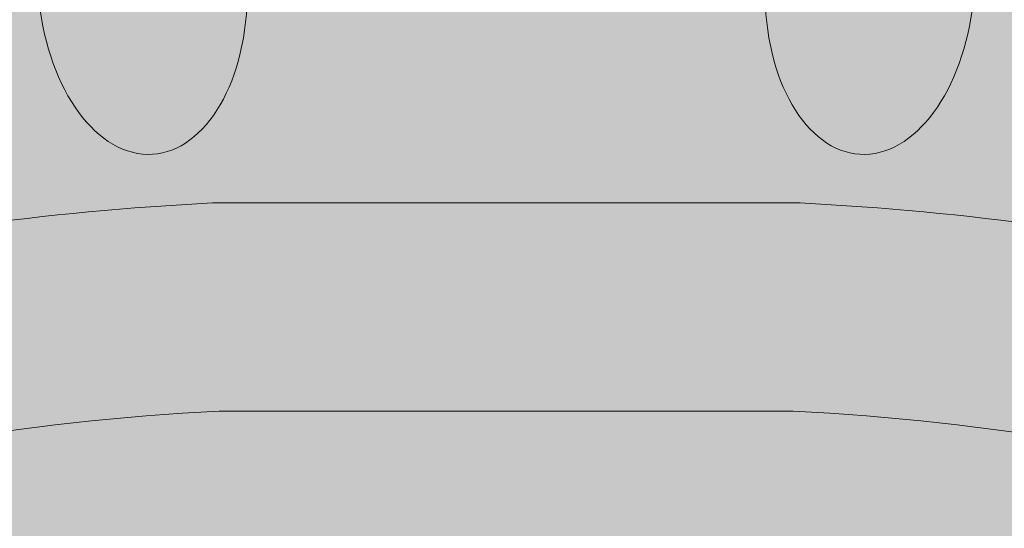
# Model space of a CAD drawing. Units: inches. Extents: x 389 to 971, y 148 to 870.
# Tile 2 of 14: x 500 to 529, y 349 to 364. Entities that reach past the tile are written whole.
import ezdxf

# ---------------------------------------------------------------- set-up
doc = ezdxf.new("R2010")
doc.units = ezdxf.units.IN
doc.header["$MEASUREMENT"] = 0
for name, color, linetype, lineweight in [('A-ANNO-DIMS', 2, 'Continuous', 18), ('C-VEHI', 8, 'Continuous', 13), ('L-GRND-BASE-PATT', 8, 'Continuous', 13)]:
    doc.layers.add(name, color=color, linetype=linetype, lineweight=lineweight)
doc.layers.add('C-VEHI-PATT', color=18, linetype='Continuous', lineweight=13, true_color=0x000000)
doc.layers.add('L-GRND-PATT', color=39, linetype='Continuous', lineweight=13, true_color=0x603913)
doc.styles.get("Standard").update_dxf_attribs({"font": 'arial.ttf'})
doc.dimstyles.get("Standard").update_dxf_attribs({"dimtxt": 8, "dimasz": 8, "dimexe": 0.18, "dimexo": 0.0625, "dimgap": 0.09, "dimtad": 0, "dimtih": 1, "dimtoh": 1, "dimdec": 0, "dimzin": 0, "dimdsep": 46, "dimlunit": 3, "dimtxsty": 'Standard', "dimcen": 0.09, "dimadec": 0, "dimazin": 0, "dimtfac": 1, "dimtdec": 0, "dimtofl": 0, "dimtmove": 0, "dimatfit": 3, "dimfxl": 1, "dimtolj": 1, "dimtzin": 0, "dimarcsym": 0})

# ---------------------------------------------------------------- blocks, each defined once
blk = doc.blocks.new('*U7')
for p, q in [((58.9167604809788, -10.77488335095668), (58.9167604809788, 10.77488335095617)), ((66.55009204259746, -10.5288681329018), (66.55009204259746, 10.52886813290129))]:
    blk.add_line(p, q)
for centre, major_axis, ratio, start_param, end_param in [((135.2911776514449, 5.387441675478555), (2.2715e-12, 81.77258453065997), 0.8423038695439563, 1.245306111696802, 1.507880129813836), ((134.4003789125686, 5.387441675477674), (4.276e-13, -89.7774543484738), 0.84230386954398, 4.44948196380473, 4.652344057257214), ((50.7902773840875, 13.33772416300607), (6.340077547122382, -0.356608581037027), 0.6038335755719145, -1.39555193967809, 1.581314658479915), ((134.4003789125684, -5.387441675478584), (4.2949e-12, -89.77745434847827), 0.8423038695439354, -1.510751403667474, -1.307889310215002), ((135.2911776514465, -5.387441675480715), (3.2038e-12, -81.77258453066244), 0.8423038695439492, -1.50788012981387, -1.245306111696839)]:
    blk.add_ellipse(centre, major_axis=major_axis, ratio=ratio, start_param=start_param, end_param=end_param)
at = {"extrusion": (0, 0, -1)}
blk.add_ellipse((50.7902773840875, -13.33772416300655), major_axis=(6.340077547122382, 0.3566085810370246), ratio=0.6038335755719145, start_param=-1.39555193967809, end_param=1.581314658479915, dxfattribs=at)
blk = doc.blocks.new('*D53')
at = {"layer": 'A-ANNO-DIMS', "color": 0, "lineweight": -2, "transparency": 16777216}
for p, q in [((397.8910240000004, 396.9189020000002), (397.8910240000004, 404.9189020000001)), ((690.1535240000002, 388.9189020000003), (397.7110240000004, 388.9189020000002)), ((690.1535240000002, 376.9189020000001), (397.7110240000005, 376.9189020000001)), ((397.8910240000005, 368.9189020000001), (397.8910240000005, 360.918902))]:
    blk.add_line(p, q, dxfattribs=at)
at = {"layer": 'A-ANNO-DIMS', "color": 0, "transparency": 16777216}
for points in [[(396.5576906666671, 396.9189020000002), (399.2243573333337, 396.9189020000002), (397.8910240000004, 388.9189020000002)], [(396.5576906666671, 368.9189020000001), (399.2243573333338, 368.9189020000001), (397.8910240000005, 376.9189020000001)]]:
    blk.add_solid(points, dxfattribs=at)
at = {"layer": 'Defpoints', "color": 0, "transparency": 16777216}
for p in [(397.8910240000004, 388.9189020000002), (690.2160240000001, 388.9189020000003), (690.2160240000001, 376.9189020000001)]:
    blk.add_point(p, dxfattribs=at)
at = {"layer": 'A-ANNO-DIMS', "color": 0, "transparency": 16777216, "insert": (397.8910240000004, 382.9189019999999), "char_height": 8, "attachment_point": 5}
blk.add_mtext('\\A1;12', dxfattribs=at)

msp = doc.modelspace()

# ---------------------------------------------------------------- hatches: boundary and pattern name
at = {"layer": 'C-VEHI-PATT'}
h = msp.add_hatch(color=256, dxfattribs=at)
h.dxf.hatch_style = 1
edge = h.paths.add_edge_path()
edge.add_ellipse((550.9021553826709, 381.4331108862803), major_axis=(-43.99405423656321, 1.9369e-12), ratio=0.8423038695439613, start_angle=-29.43856959797762, end_angle=1.8189894035458565e-12, ccw=False)
edge.add_line((514.3535105156315, 402.059641051582), (514.3535105156315, 404.7525403567118))
edge.add_ellipse((514.3535105156316, 404.2643898676136), major_axis=(0.5795420236673633, 2e-16), ratio=0.8423038695437671, start_angle=90.00000000001334, end_angle=127.9331304598466)
edge.add_line((514.0354569934393, 404.6724605914631), (509.5535496243029, 402.1940957519602))
edge.add_ellipse((473.3138688667988, 564.9222417143382), major_axis=(196.5636751472093, 8.4793e-12), ratio=0.8423038695439335, start_angle=-80.7434339928015, end_angle=-77.44506735586577, ccw=False)
edge.add_ellipse((535.9119176052684, 201.7546502845751), major_axis=(239.1273775699096, 1.008988e-10), ratio=0.842303869543627, start_angle=100.2095389971183, end_angle=102.4446272934191)
edge.add_ellipse((979.5722266908713, 375.4013592680145), major_axis=(-488.2195497741742, 7.7268e-12), ratio=0.842303869543895, start_angle=-2.863714607837472, end_angle=2.198540565955285)
edge.add_ellipse((510.1338164488812, 299.4839331720496), major_axis=(70.3178640738586, 3.814e-12), ratio=0.8423038695439212, start_angle=94.08241069114638, end_angle=107.71995322274631, ccw=False)
edge.add_line((505.914122382133, 358.6062023341113), (522.79289864913, 358.606202334111))
edge.add_ellipse((518.5732045823792, 299.4839331720493), major_axis=(-70.31786407385354, 1.4408e-12), ratio=0.8423038695439844, start_angle=252.2800467772501, end_angle=265.91758930884987, ccw=False)
edge.add_ellipse((49.13479434038987, 375.4013592680261), major_axis=(-488.2195497741754, 2.5232e-12), ratio=0.8423038695439587, start_angle=177.8014594340444, end_angle=182.8637146078372)
edge.add_ellipse((492.795103425985, 201.7546502845724), major_axis=(239.12737756976, 4.82267e-11), ratio=0.8423038695441539, start_angle=77.5553727065425, end_angle=79.79046100284327)
edge.add_ellipse((555.3931521644682, 564.9222417143374), major_axis=(-196.5636751472384, 3.62381e-11), ratio=0.8423038695438114, start_angle=77.4450673558726, end_angle=80.74343399280832, ccw=False)
edge.add_line((519.1534714069603, 402.19409575196), (514.671564037824, 404.6724605914631))
edge.add_ellipse((514.3535105156316, 404.2643898676136), major_axis=(0.5795420236673633, 2e-16), ratio=0.8423038695437671, start_angle=52.06686954015338, end_angle=90.00000000001334)
edge.add_line((514.3535105156315, 404.7525403567118), (514.3535105156315, 402.0596410515821))
edge.add_ellipse((477.8048656485917, 381.4331108862812), major_axis=(-43.99405423656326, 6.67e-13), ratio=0.8423038695439753, start_angle=180.0000000000002, end_angle=209.4385695979796, ccw=False)
edge.add_line((521.7989198851549, 381.4331108862806), (521.7989198851549, 379.5923831537828))
edge.add_line((521.7989198851549, 379.5923831537828), (523.2258361412675, 379.5923831537828))
edge.add_ellipse((523.0896049791924, 379.1042326646847), major_axis=(0.5795420236669786, 3.601e-13), ratio=0.8423038695443263, start_angle=45.519789117397124, end_angle=89.99999999996442, ccw=False)
edge.add_line((523.4589887688404, 379.4803801228631), (527.8015488731598, 376.4548385069232))
edge.add_line((527.8015488731598, 376.4548385069232), (527.8015488731597, 364.8548231745798))
edge.add_ellipse((524.8002343791572, 364.9712406163019), major_axis=(0.279312372030448, 4.96584264291768), ratio=0.6038335755719146, start_angle=106.34259195429831, end_angle=270.9979857249735, ccw=False)
edge.add_line((521.7989198851548, 364.2715269884119), (521.7989198851549, 381.4331108862806))
edge.add_ellipse((477.8048656485917, 381.4331108862812), major_axis=(-43.99405423656326, 6.67e-13), ratio=0.8423038695439753, start_angle=180.0000000000001, end_angle=209.4385695979795)
edge.add_ellipse((550.9021553826709, 381.4331108862803), major_axis=(-43.99405423656321, 1.9369e-12), ratio=0.8423038695439613, start_angle=-29.43856959797755, end_angle=1.8539e-12)
edge.add_line((506.9081011461076, 381.43311088628), (506.9081011461074, 364.2715269884121))
edge.add_ellipse((503.9067866521049, 364.9712406163021), major_axis=(-0.2793123720310282, 4.965842642917721), ratio=0.6038335755718928, start_angle=89.00201427501901, end_angle=253.6574080456941, ccw=False)
edge.add_line((500.9054721581025, 364.8548231745812), (500.9054721581025, 376.4548385069235))
edge.add_line((500.9054721581025, 376.4548385069235), (505.3530060491612, 379.5535172937331))
edge.add_ellipse((505.61741605207, 379.1042326646849), major_axis=(-0.5795420236672051, 1.236e-13), ratio=0.842303869543997, start_angle=-89.99999999998778, end_angle=-45.51978911742469, ccw=False)
edge.add_line((505.61741605207, 379.5923831537831), (506.9081011461076, 379.5923831537831))
edge.add_line((506.9081011461076, 379.5923831537831), (506.9081011461076, 381.43311088628))
h = msp.add_hatch(color=256, dxfattribs=at)
h.dxf.hatch_style = 1
edge = h.paths.add_edge_path()
edge.add_ellipse((550.9021553826709, 381.4331108862803), major_axis=(-43.99405423656321, 1.9369e-12), ratio=0.8423038695439613, start_angle=-17.01851281727818, end_angle=1.8189894035458565e-12, ccw=False)
edge.add_line((509.5535496243029, 394.0892586662828), (509.5535496243029, 402.1940957519602))
edge.add_ellipse((473.3138688667988, 564.9222417143382), major_axis=(196.5636751472093, 8.4793e-12), ratio=0.8423038695439335, start_angle=-80.7434339928015, end_angle=-77.44506735586577, ccw=False)
edge.add_ellipse((535.9119176052684, 201.7546502845751), major_axis=(239.1273775699096, 1.008988e-10), ratio=0.842303869543627, start_angle=100.2095389971183, end_angle=102.4446272934191)
edge.add_ellipse((979.5722266908713, 375.4013592680145), major_axis=(-488.2195497741742, 7.7268e-12), ratio=0.842303869543895, start_angle=-2.863714607837472, end_angle=2.198540565955285)
edge.add_ellipse((510.1338164488812, 299.4839331720496), major_axis=(70.3178640738586, 3.814e-12), ratio=0.8423038695439212, start_angle=94.08241069114638, end_angle=107.71995322274631, ccw=False)
edge.add_line((505.914122382133, 358.6062023341113), (509.5535496243029, 358.6062023341112))
edge.add_line((509.5535496243029, 358.6062023341112), (509.5535496243029, 394.0892586662828))
edge.add_ellipse((550.9021553826709, 381.4331108862803), major_axis=(-43.99405423656321, 1.9369e-12), ratio=0.8423038695439613, start_angle=-17.01851281727824, end_angle=1.8539e-12)
edge.add_line((506.9081011461076, 381.43311088628), (506.9081011461074, 364.2715269884121))
edge.add_ellipse((503.9067866521049, 364.9712406163021), major_axis=(-0.2793123720310282, 4.965842642917721), ratio=0.6038335755718928, start_angle=89.00201427501901, end_angle=253.6574080456941, ccw=False)
edge.add_line((500.9054721581025, 364.8548231745812), (500.9054721581025, 376.4548385069235))
edge.add_line((500.9054721581025, 376.4548385069235), (505.3172273641584, 379.5285896248376))
edge.add_ellipse((505.61741605207, 379.1042326646849), major_axis=(-0.5795420236672051, 1.236e-13), ratio=0.842303869543997, start_angle=-89.99999999998778, end_angle=-45.51978911742469, ccw=False)
edge.add_line((505.61741605207, 379.5923831537831), (506.9081011461076, 379.5923831537831))
edge.add_line((506.9081011461076, 379.5923831537831), (506.9081011461076, 381.43311088628))
h = msp.add_hatch(color=256, dxfattribs=at)
h.dxf.hatch_style = 1
edge = h.paths.add_edge_path()
edge.add_ellipse((492.795103425985, 201.7546502845724), major_axis=(239.12737756976, 4.82267e-11), ratio=0.8423038695441539, start_angle=77.5553727065425, end_angle=79.79046100284327)
edge.add_ellipse((555.3931521644682, 564.9222417143374), major_axis=(-196.5636751472384, 3.62381e-11), ratio=0.8423038695438114, start_angle=77.4450673558726, end_angle=80.74343399280832, ccw=False)
edge.add_line((519.1534714069603, 402.19409575196), (519.1534714069603, 394.0892586662818))
edge.add_ellipse((477.8048656485917, 381.4331108862812), major_axis=(-43.99405423656326, 6.67e-13), ratio=0.8423038695439753, start_angle=180.0000000000002, end_angle=197.0185128172791, ccw=False)
edge.add_line((521.7989198851549, 381.4331108862806), (521.7989198851549, 379.5923831537828))
edge.add_line((521.7989198851549, 379.5923831537828), (523.1794038652976, 379.5923831537828))
edge.add_ellipse((523.0896049791924, 379.1042326646847), major_axis=(0.5795420236669786, 3.601e-13), ratio=0.8423038695443263, start_angle=45.519789117397124, end_angle=89.99999999996442, ccw=False)
edge.add_line((523.4589887688405, 379.480380122863), (527.8015488731598, 376.4548385069232))
edge.add_line((527.8015488731598, 376.4548385069232), (527.8015488731597, 364.8548231745798))
edge.add_ellipse((524.8002343791572, 364.9712406163019), major_axis=(0.279312372030448, 4.96584264291768), ratio=0.6038335755719146, start_angle=106.34259195429831, end_angle=270.9979857249735, ccw=False)
edge.add_line((521.7989198851548, 364.2715269884119), (521.7989198851549, 381.4331108862806))
edge.add_ellipse((477.8048656485917, 381.4331108862812), major_axis=(-43.99405423656326, 6.67e-13), ratio=0.8423038695439753, start_angle=180.0000000000001, end_angle=197.018512817279)
edge.add_line((519.1534714069603, 394.0892586662818), (519.1534714069603, 358.6062023341111))
edge.add_line((519.1534714069603, 358.6062023341111), (522.79289864913, 358.606202334111))
edge.add_ellipse((518.5732045823792, 299.4839331720493), major_axis=(-70.31786407385354, 1.4408e-12), ratio=0.8423038695439844, start_angle=252.2800467772501, end_angle=265.91758930884987, ccw=False)
edge.add_ellipse((49.13479434038987, 375.4013592680261), major_axis=(-488.2195497741754, 2.5232e-12), ratio=0.8423038695439587, start_angle=177.8014594340444, end_angle=182.8637146078372)
h = msp.add_hatch(color=256, dxfattribs=at)
h.dxf.hatch_style = 1
edge = h.paths.add_edge_path(flags=16)
edge.add_ellipse((3386.011413077446, 329.726312794031), major_axis=(-2896.629999631248, 1.069454e-10), ratio=0.8423038695494893, start_angle=-0.1208973690315247, end_angle=0.3640763488915013, ccw=False)
edge.add_line((489.3905023836935, 335.8383575186984), (486.2179253655185, 346.1978202249628))
edge.add_ellipse((8782.002602781096, 354.247254279773), major_axis=(-8295.790181758603, 9.87839e-10), ratio=0.8423038695486498, start_angle=0.0555943135052214, end_angle=0.3777641939157137)
edge.add_line((486.4665645878948, 299.5520931219791), (489.4638383140943, 311.3204429697198))
edge = h.paths.add_edge_path(flags=16)
edge.add_ellipse((512.1608573463288, 287.5825181681774), major_axis=(62.33048198263887, 2.0798e-12), ratio=0.8423038695439498, start_angle=94.8700695971331, end_angle=112.791914877584)
edge.add_line((491.3642517254777, 337.0752369161335), (489.6529508739416, 349.9015767089268))
edge.add_ellipse((510.1338164488795, 298.7862183048575), major_axis=(64.04807894948699, 3.9006e-12), ratio=0.8423038695439252, start_angle=94.27742096304979, end_angle=111.83495379670401, ccw=False)
edge.add_line((506.1068129054811, 352.6274231954524), (522.600208125781, 352.6274231954521))
edge.add_ellipse((518.5732045823798, 298.7862183048586), major_axis=(64.04807894948067, 3.24e-14), ratio=0.8423038695439885, start_angle=68.16504620328948, end_angle=85.72257903694378, ccw=False)
edge.add_line((539.05407015732, 349.9015767089259), (537.3427693057835, 337.0752369161327))
edge.add_ellipse((516.5461636849332, 287.5825181681899), major_axis=(62.33048198262021, 1.5954e-12), ratio=0.8423038695439995, start_angle=67.20808512240782, end_angle=85.12993040286212)
edge.add_line((521.0080028322477, 339.9490379899644), (507.6990181990146, 339.9490379899646))
edge = h.paths.add_edge_path(flags=16)
edge.add_ellipse((514.3535105156315, 391.3730654902235), major_axis=(-115.1512533244504, 1.8736e-12), ratio=0.8423038695439684, start_angle=76.4018653097696, end_angle=103.5981346902308)
edge.add_line((537.3427693057832, 296.3333211885938), (537.342769305783, 281.5897392316151))
edge.add_ellipse((514.3535105156313, 376.6294835332447), major_axis=(-115.1512533244486, 9.02e-13), ratio=0.8423038695439828, start_angle=76.40186530976922, end_angle=103.59813469023032, ccw=False)
edge.add_line((491.3642517254773, 281.5897392316156), (491.3642517254774, 296.3333211885945))
edge = h.paths.add_edge_path()
edge.add_ellipse((8782.002602781105, 354.2472542798386), major_axis=(-8296.949265805946, 5.39345e-11), ratio=0.8423038695428886, start_angle=0.3838667787920247, end_angle=0.5282714718170651)
edge.add_ellipse((8782.002602781105, 354.2472542798386), major_axis=(-8296.949265805946, 5.39345e-11), ratio=0.8423038695428886, start_angle=0.5282714718170651, end_angle=0.6465540970606384)
edge.add_ellipse((488.1158467995968, 260.6509346628684), major_axis=(2.318168094668909, 7.48e-14), ratio=0.8423038695439647, start_angle=180.6465540970884, end_angle=269.9999999999081)
edge.add_line((488.115846799593, 258.6983327064755), (491.3642517254771, 258.6983327064753))
edge.add_line((491.3642517254771, 258.6983327064753), (491.3642517254771, 274.201106836649))
edge.add_ellipse((493.6824198201462, 273.9438556676354), major_axis=(-2.318168094668919, 1.896e-13), ratio=0.8423038695439611, start_angle=-89.99999999999523, end_angle=4.718003765447065e-12, ccw=False)
edge.add_line((493.6824198201462, 275.8964576240284), (535.3300149439905, 275.8964576240277))
edge.add_ellipse((535.024601211114, 273.9438556676347), major_axis=(2.318168094668976, 2.946e-13), ratio=0.8423038695439647, start_angle=-7.275957614183426e-12, end_angle=89.99999999998943, ccw=False)
edge.add_line((537.342769305783, 273.9438556676347), (537.3427693057827, 258.698332706474))
edge.add_line((537.3427693057827, 258.698332706474), (540.591174231666, 258.6983327064739))
edge.add_ellipse((540.5911742316634, 260.6509346628669), major_axis=(-2.318168094668839, 2.143e-13), ratio=0.8423038695440144, start_angle=90.00000000008203, end_angle=179.3534459029346)
edge.add_ellipse((-7753.295581726658, 354.2472542799028), major_axis=(-8296.949265782761, 2.068448e-10), ratio=0.8423038695442414, start_angle=179.3534459029388, end_angle=179.3813568036815)
edge.add_ellipse((-7753.295581726658, 354.2472542799028), major_axis=(-8296.949265782761, 2.068448e-10), ratio=0.8423038695442414, start_angle=179.3813568036815, end_angle=179.4717285281828)
edge.add_ellipse((-7753.295581726658, 354.2472542799028), major_axis=(-8296.949265782761, 2.068448e-10), ratio=0.8423038695442414, start_angle=179.4717285281828, end_angle=179.6161332212082)
edge.add_ellipse((-7753.295581726658, 354.2472542799028), major_axis=(-8296.949265782761, 2.068448e-10), ratio=0.8423038695442414, start_angle=179.6161332212082, end_angle=180.090229088595)
edge.add_ellipse((-7753.295581726658, 354.2472542799028), major_axis=(-8296.949265782761, 2.068448e-10), ratio=0.8423038695442414, start_angle=180.090229088595, end_angle=180.134986576859)
edge.add_ellipse((129.8867725257751, 372.4897205359271), major_axis=(-413.7373561031673, 2.44623e-11), ratio=0.8423038695441432, start_angle=180.1806905311865, end_angle=182.1799503136479)
edge.add_ellipse((129.8867725257751, 372.4897205359271), major_axis=(-413.7373561031673, 2.44623e-11), ratio=0.8423038695441432, start_angle=182.1799503136479, end_angle=183.6504275857017)
edge.add_ellipse((492.7951034259847, 196.3854951855023), major_axis=(245.3971626940514, 1.422861e-10), ratio=0.8423038695444116, start_angle=76.21947101046817, end_angle=77.87403444768196)
edge.add_ellipse((49.13479434038987, 375.4013592680261), major_axis=(-488.2195497741754, 2.5232e-12), ratio=0.8423038695439587, start_angle=177.8014594340445, end_angle=182.8637146078372, ccw=False)
edge.add_ellipse((518.5732045823792, 299.4839331720493), major_axis=(-70.31786407385354, 1.4408e-12), ratio=0.8423038695439844, start_angle=252.2800467772501, end_angle=265.9175893088498)
edge.add_line((522.79289864913, 358.606202334111), (505.9141223821329, 358.6062023341113))
edge.add_ellipse((510.1338164488812, 299.4839331720496), major_axis=(70.3178640738586, 3.814e-12), ratio=0.8423038695439212, start_angle=94.08241069114636, end_angle=107.7199532227462)
edge.add_ellipse((979.5722266908713, 375.4013592680145), major_axis=(-488.2195497741742, 7.7268e-12), ratio=0.842303869543895, start_angle=-2.863714607837494, end_angle=2.198540565955284, ccw=False)
edge.add_ellipse((535.9119176052733, 196.3854951855018), major_axis=(-245.3971626940985, 1.013648e-10), ratio=0.8423038695442548, start_angle=-77.87403444769295, end_angle=-76.2194710104792)
edge.add_ellipse((898.8202485054873, 372.489720535918), major_axis=(413.7373561031672, 1.26113e-11), ratio=0.8423038695441164, start_angle=176.3495724142985, end_angle=177.8200496863523)
edge.add_ellipse((898.8202485054873, 372.489720535918), major_axis=(413.7373561031672, 1.26113e-11), ratio=0.8423038695441164, start_angle=177.8200496863523, end_angle=179.8643876095591)
edge.add_ellipse((8782.002602781105, 354.2472542798386), major_axis=(-8296.949265805946, 5.39345e-11), ratio=0.8423038695428886, start_angle=-0.1349865768573029, end_angle=-0.090229088593484)
edge.add_ellipse((8782.002602781105, 354.2472542798386), major_axis=(-8296.949265805946, 5.39345e-11), ratio=0.8423038695428886, start_angle=-0.090229088593484, end_angle=0.3838667787920247)
edge = h.paths.add_edge_path(flags=16)
edge.add_ellipse((-2357.304392046186, 329.7263127941099), major_axis=(2896.629999631251, 5.35614e-11), ratio=0.8423038695445265, start_angle=-0.3640763488920631, end_angle=0.1208973690309369)
edge.add_line((539.3165186475693, 335.8383575187012), (542.4890956657468, 346.1978202249727))
edge.add_ellipse((-7753.295581749842, 354.2472542800017), major_axis=(8295.790181758617, 3.2664368e-09), ratio=0.8423038695525207, start_angle=-0.37776419393310334, end_angle=-0.055594313522590255, ccw=False)
edge.add_line((542.240456443367, 299.5520931219743), (539.2431827171666, 311.3204429697195))
h = msp.add_hatch(color=256, dxfattribs=at)
h.dxf.hatch_style = 1
edge = h.paths.add_edge_path()
edge.add_ellipse((501.0307058076602, 393.6297666969722), major_axis=(-21.47347468096764, 1.6558e-12), ratio=0.8423038695440453, start_angle=89.60329014002599, end_angle=108.66749549260749, ccw=False)
edge.add_line((500.9054721581025, 375.5428834777413), (500.9054721581025, 364.8548231745812))
edge.add_ellipse((503.9067866521049, 364.9712406163021), major_axis=(-0.2793123720310282, 4.965842642917721), ratio=0.6038335755718928, start_angle=89.0020142750189, end_angle=253.657408045694)
edge.add_line((506.9081011461074, 364.2715269884121), (506.9081011461076, 376.2332584772061))
h = msp.add_hatch(color=256, dxfattribs=at)
h.dxf.hatch_style = 1
edge = h.paths.add_edge_path()
edge.add_ellipse((501.0307058076602, 393.6297666969722), major_axis=(-21.47347468096764, 1.6558e-12), ratio=0.8423038695440453, start_angle=89.60329014002599, end_angle=108.66749549260749, ccw=False)
edge.add_line((500.9054721581025, 375.5428834777413), (500.9054721581025, 364.8548231745812))
edge.add_ellipse((503.9067866521049, 364.9712406163021), major_axis=(-0.2793123720310282, 4.965842642917721), ratio=0.6038335755718928, start_angle=89.0020142750189, end_angle=253.657408045694)
edge.add_line((506.9081011461074, 364.2715269884121), (506.9081011461076, 376.2332584772061))
h = msp.add_hatch(color=256, dxfattribs=at)
h.dxf.hatch_style = 1
edge = h.paths.add_edge_path()
edge.add_ellipse((527.6763152236027, 393.629766696972), major_axis=(-21.47347468097092, 1.1981e-12), ratio=0.8423038695439196, start_angle=71.33250450739882, end_angle=90.39670985998049, ccw=False)
edge.add_line((521.7989198851549, 376.2332584772058), (521.7989198851548, 364.2715269884119))
edge.add_ellipse((524.8002343791572, 364.9712406163019), major_axis=(0.279312372030448, 4.96584264291768), ratio=0.6038335755719146, start_angle=106.3425919542983, end_angle=270.9979857249735)
edge.add_line((527.8015488731597, 364.8548231745798), (527.8015488731598, 375.5428834777409))
h = msp.add_hatch(color=256, dxfattribs=at)
h.dxf.hatch_style = 1
edge = h.paths.add_edge_path()
edge.add_ellipse((527.6763152236027, 393.629766696972), major_axis=(-21.47347468097092, 1.1981e-12), ratio=0.8423038695439196, start_angle=71.33250450739882, end_angle=90.39670985998049, ccw=False)
edge.add_line((521.7989198851549, 376.2332584772058), (521.7989198851548, 364.2715269884119))
edge.add_ellipse((524.8002343791572, 364.9712406163019), major_axis=(0.279312372030448, 4.96584264291768), ratio=0.6038335755719146, start_angle=106.3425919542983, end_angle=270.9979857249735)
edge.add_line((527.8015488731597, 364.8548231745798), (527.8015488731598, 375.5428834777409))
h = msp.add_hatch(color=256, dxfattribs=at)
h.dxf.hatch_style = 1
edge = h.paths.add_edge_path()
edge.add_ellipse((518.5732045823798, 298.7862183048586), major_axis=(64.04807894948067, 3.24e-14), ratio=0.8423038695439885, start_angle=68.16504620328955, end_angle=85.72257903694374)
edge.add_line((522.600208125781, 352.6274231954521), (506.106812905481, 352.6274231954524))
edge.add_ellipse((510.1338164488795, 298.7862183048575), major_axis=(64.04807894948699, 3.9006e-12), ratio=0.8423038695439252, start_angle=94.2774209630498, end_angle=111.834953796704)
edge.add_line((489.6529508739416, 349.9015767089268), (491.3642517254777, 337.0752369161335))
edge.add_ellipse((512.1608573463288, 287.5825181681774), major_axis=(62.33048198263887, 2.0798e-12), ratio=0.8423038695439498, start_angle=94.87006959713312, end_angle=112.79191487758399, ccw=False)
edge.add_line((507.6990181990146, 339.9490379899646), (521.0080028322477, 339.9490379899644))
edge.add_ellipse((516.5461636849332, 287.5825181681899), major_axis=(62.33048198262021, 1.5954e-12), ratio=0.8423038695439995, start_angle=67.2080851224078, end_angle=85.1299304028621, ccw=False)
edge.add_line((537.3427693057835, 337.0752369161327), (539.05407015732, 349.9015767089259))
at = {"layer": 'L-GRND-BASE-PATT'}
h = msp.add_hatch(color=256, dxfattribs=at)
h.dxf.hatch_style = 1
edge = h.paths.add_edge_path(flags=16)
edge.add_ellipse((8782.002602781105, 354.2472542798386), major_axis=(-8296.949265805946, 5.39345e-11), ratio=0.8423038695428886, start_angle=-0.0902290885933894, end_angle=0.3838667787920258, ccw=False)
edge.add_ellipse((485.0533369751568, 368.2895347624687), major_axis=(-1.159084047334488, 1.838e-13), ratio=0.8423038695439892, start_angle=9.094947017729282e-12, end_angle=90.00000000000898, ccw=False)
edge.add_line((483.8942529278224, 368.2895347624687), (483.8942529278225, 387.6039063360424))
edge.add_ellipse((485.0533369751571, 387.2465553762829), major_axis=(1.159084047334488, 1.838e-13), ratio=0.8423038695439892, start_angle=89.99999999999102, end_angle=179.9999999999909, ccw=False)
edge.add_line((485.0533369751572, 388.2228563544795), (485.5047440247956, 388.2228563544795))
edge.add_ellipse((898.8202485054873, 372.489720535918), major_axis=(413.7373561031672, 1.26113e-11), ratio=0.8423038695441164, start_angle=176.3495724142986, end_angle=177.8200496863524, ccw=False)
edge.add_ellipse((535.9119176052733, 196.3854951855018), major_axis=(-245.3971626940985, 1.013648e-10), ratio=0.8423038695442548, start_angle=-77.87403444769302, end_angle=-76.2194710104792, ccw=False)
edge.add_ellipse((535.9119176052684, 201.7546502845751), major_axis=(239.1273775699096, 1.008988e-10), ratio=0.842303869543627, start_angle=100.20953899711827, end_angle=102.44462729341922, ccw=False)
edge.add_ellipse((473.3138688667988, 564.9222417143382), major_axis=(196.5636751472093, 8.4793e-12), ratio=0.8423038695439335, start_angle=-80.74343399280163, end_angle=-77.44506735586587)
edge.add_line((509.5535496243029, 402.1940957519602), (514.3535105156315, 404.8483349684994))
edge.add_line((514.3535105156315, 404.8483349684994), (514.3535105156315, 404.7971763262221))
edge.add_ellipse((514.3535105156316, 404.2643898676136), major_axis=(0.5795420236673633, 2e-16), ratio=0.8423038695437671, start_angle=52.06686954015339, end_angle=90.00000000001342, ccw=False)
edge.add_line((514.671564037824, 404.672460591463), (519.1534714069603, 402.19409575196))
edge.add_ellipse((555.3931521644682, 564.9222417143374), major_axis=(-196.5636751472384, 3.62381e-11), ratio=0.8423038695438114, start_angle=77.44506735587258, end_angle=80.74343399280833)
edge.add_ellipse((492.795103425985, 201.7546502845724), major_axis=(239.12737756976, 4.82267e-11), ratio=0.8423038695441539, start_angle=77.55537270654253, end_angle=79.7904610028433, ccw=False)
edge.add_ellipse((492.7951034259847, 196.3854951855023), major_axis=(245.3971626940514, 1.422861e-10), ratio=0.8423038695444116, start_angle=76.21947101046823, end_angle=77.87403444768199, ccw=False)
edge.add_ellipse((129.8867725257751, 372.4897205359271), major_axis=(-413.7373561031673, 2.44623e-11), ratio=0.8423038695441432, start_angle=182.179950313648, end_angle=183.6504275857018, ccw=False)
edge.add_line((543.2022770064673, 388.2228563544788), (544.0779382625514, 388.2228563544787))
edge.add_ellipse((543.6536840561057, 387.2465553762822), major_axis=(-1.159084047334545, 1.527e-13), ratio=0.8423038695438989, start_angle=180.0000000000075, end_angle=270.00000000000756, ccw=False)
edge.add_line((544.8127681034401, 387.2465553762826), (544.8127681034399, 367.9321838027083))
edge.add_ellipse((543.6536840561054, 368.2895347624679), major_axis=(1.159084047334544, 7.24e-14), ratio=0.8423038695439478, start_angle=269.9999999999964, end_angle=359.9999999999964, ccw=False)
edge.add_ellipse((-7753.295581726658, 354.2472542799028), major_axis=(-8296.949265782761, 2.068448e-10), ratio=0.8423038695442414, start_angle=179.6161332212083, end_angle=180.0902290885951, ccw=False)
edge.add_line((543.3912265319653, 298.6607849184036), (544.0779382625504, 298.6607849184036))
edge.add_ellipse((543.6536840561046, 297.6844839402071), major_axis=(1.159084047334431, 1.769e-13), ratio=0.8423038695439814, start_angle=-1.1482370609883219e-11, end_angle=89.99999999999119, ccw=False)
edge.add_line((544.8127681034391, 297.684483940207), (544.8127681034387, 278.3701123666333))
edge.add_ellipse((543.6536840561043, 278.727463326393), major_axis=(-1.159084047334431, 2.574e-13), ratio=0.8423038695440306, start_angle=90.00000000001268, end_angle=180.0000000000099, ccw=False)
edge.add_line((543.6536840561045, 277.7511623481965), (543.1566278692261, 277.7511623481965))
edge.add_ellipse((-7753.295581726658, 354.2472542799028), major_axis=(-8296.949265782761, 2.068448e-10), ratio=0.8423038695442414, start_angle=179.3813568036816, end_angle=179.4717285281829, ccw=False)
edge.add_ellipse((542.4236240941387, 263.2762864208561), major_axis=(-1.738626071001761, 2.132e-13), ratio=0.8423038695439151, start_angle=179.3717627838137, end_angle=248.464756601011, ccw=False)
edge.add_ellipse((-7753.875123750511, 354.2472542780016), major_axis=(-8298.740341433751, 2.4782644722e-06), ratio=0.8423038662721074, start_angle=179.3534459200609, end_angle=179.3717628008941, ccw=False)
edge.add_ellipse((540.0116322079951, 260.6509346628677), major_axis=(-4.109243751168186, 2.384e-13), ratio=0.842303869543976, start_angle=90.0000000000635, end_angle=179.3534459029233, ccw=False)
edge.add_line((540.0116322079991, 257.1897027503593), (488.6953888232593, 257.1897027503609))
edge.add_ellipse((488.6953888232669, 260.6509346628715), major_axis=(4.10924375117072, 1.262e-13), ratio=0.8423038695439824, start_angle=180.6465540970565, end_angle=269.9999999998589, ccw=False)
edge.add_ellipse((8782.582144816053, 354.2472542821698), major_axis=(-8298.740341477976, 1.8591886369e-06), ratio=0.8423038720186145, start_angle=0.6282372290784792, end_angle=0.6465541099116194, ccw=False)
edge.add_ellipse((486.2833969371199, 263.2762864208594), major_axis=(-1.738626071002378, 2.7e-13), ratio=0.8423038695439394, start_angle=-68.46475649596817, end_angle=0.6282372161796275, ccw=False)
edge.add_ellipse((8782.002602781105, 354.2472542798386), major_axis=(-8296.949265805946, 5.39345e-11), ratio=0.8423038695428886, start_angle=0.5282714718171064, end_angle=0.6465540970606867, ccw=False)
edge.add_line((485.5503931620382, 277.7511623481972), (484.6290827687102, 277.7511623481972))
edge.add_ellipse((485.0533369751559, 278.7274633263938), major_axis=(-1.159084047334545, 3.11e-13), ratio=0.8423038695439968, start_angle=1.5404566511278972e-11, end_angle=90.000000000012, ccw=False)
edge.add_line((483.8942529278214, 278.7274633263938), (483.8942529278216, 298.0418348999672))
edge.add_ellipse((485.053336975156, 297.6844839402078), major_axis=(1.159084047334488, 1.025e-13), ratio=0.8423038695440382, start_angle=89.99999999999488, end_angle=179.9999999999949, ccw=False)
edge = h.paths.add_edge_path(flags=0)
edge.add_ellipse((8782.002602781096, 354.247254279773), major_axis=(-8295.790181758603, 9.87839e-10), ratio=0.8423038695486498, start_angle=0.05559431350519617, end_angle=0.37776419391582294, ccw=False)
edge.add_line((486.2179253655185, 346.1978202249628), (489.3905023836935, 335.8383575186984))
edge.add_ellipse((3386.011413077446, 329.726312794031), major_axis=(-2896.629999631248, 1.069454e-10), ratio=0.8423038695494893, start_angle=-0.1208973690315206, end_angle=0.3640763488915184)
edge.add_line((489.4638383140943, 311.3204429697198), (486.4665645878948, 299.5520931219791))
edge = h.paths.add_edge_path(flags=0)
edge.add_ellipse((514.3535105156315, 391.3730654902235), major_axis=(-115.1512533244504, 1.8736e-12), ratio=0.8423038695439684, start_angle=76.4018653097696, end_angle=103.5981346902308)
edge.add_line((537.3427693057832, 296.3333211885938), (537.342769305783, 281.5897392316151))
edge.add_ellipse((514.3535105156313, 376.6294835332447), major_axis=(-115.1512533244486, 9.02e-13), ratio=0.8423038695439828, start_angle=76.40186530976922, end_angle=103.59813469023032, ccw=False)
edge.add_line((491.3642517254773, 281.5897392316156), (491.3642517254774, 296.3333211885945))
edge = h.paths.add_edge_path(flags=0)
edge.add_line((491.3642517254777, 337.0752369161334), (489.6529508739416, 349.9015767089268))
edge.add_ellipse((510.1338164488795, 298.7862183048575), major_axis=(64.04807894948699, 3.9006e-12), ratio=0.8423038695439252, start_angle=94.27742096304979, end_angle=111.83495379670401, ccw=False)
edge.add_line((506.106812905481, 352.6274231954524), (522.600208125781, 352.6274231954521))
edge.add_ellipse((518.5732045823798, 298.7862183048586), major_axis=(64.04807894948067, 3.24e-14), ratio=0.8423038695439885, start_angle=68.16504620328948, end_angle=85.72257903694378, ccw=False)
edge.add_line((539.05407015732, 349.9015767089259), (537.3427693057835, 337.0752369161327))
edge.add_ellipse((516.5461636849332, 287.5825181681899), major_axis=(62.33048198262021, 1.5954e-12), ratio=0.8423038695439995, start_angle=67.20808512240782, end_angle=85.12993040286212)
edge.add_line((521.0080028322477, 339.9490379899644), (507.6990181990146, 339.9490379899646))
edge.add_ellipse((512.1608573463288, 287.5825181681774), major_axis=(62.33048198263887, 2.0798e-12), ratio=0.8423038695439498, start_angle=94.8700695971331, end_angle=112.791914877584)
edge = h.paths.add_edge_path(flags=0)
edge.add_ellipse((493.6824198201462, 273.9438556676354), major_axis=(-2.318168094668919, 1.896e-13), ratio=0.8423038695439611, start_angle=-89.99999999999523, end_angle=4.718003765447065e-12, ccw=False)
edge.add_line((493.6824198201462, 275.8964576240284), (535.3743409680425, 275.8964576240277))
edge.add_ellipse((535.024601211114, 273.9438556676347), major_axis=(2.318168094668976, 2.946e-13), ratio=0.8423038695439647, start_angle=-7.275957614183426e-12, end_angle=89.99999999998943, ccw=False)
edge.add_line((537.342769305783, 273.9438556676347), (537.3427693057827, 258.698332706474))
edge.add_line((537.3427693057827, 258.698332706474), (540.5911742316662, 258.6983327064739))
edge.add_ellipse((540.5911742316634, 260.6509346628669), major_axis=(-2.318168094668839, 2.143e-13), ratio=0.8423038695440144, start_angle=90.00000000008203, end_angle=179.3534459029346)
edge.add_line((540.5911742316662, 258.6983327064739), (487.7691399811528, 258.6983327064755))
edge.add_ellipse((488.1158467995968, 260.6509346628684), major_axis=(2.318168094668909, 7.48e-14), ratio=0.8423038695439647, start_angle=180.6465540970884, end_angle=269.9999999999081)
edge.add_line((488.1158467995931, 258.6983327064755), (491.3642517254771, 258.6983327064754))
edge.add_line((491.3642517254771, 258.6983327064754), (491.3642517254771, 274.2384428182294))
h.paths.add_polyline_path([(746.1375687288224, 327.3223047166553), (750.1400147212453, 327.3223047166553), (750.1400147212453, 326.2830696147227), (798.1693712998389, 326.2830696147227), (798.1693712998389, 327.3223047166553), (802.1718172922616, 327.3223047166553), (802.1718172922616, 309.9783792024682, -0.1904762075443491), (746.1375687288224, 309.9783668090107)], flags=16)
h.paths.add_polyline_path([(782.1595875801748, 313.5684994305933), (782.1595893317732, 309.0414930416419, -0.0496282101666581), (766.1497986905329, 309.0414910503953), (766.1498004421323, 313.5684994305933)], flags=0)
h.paths.add_polyline_path([(755.1858908233534, 344.9352232902417), (755.1858908233534, 373.916311072083), (788.1243995226009, 373.916311072083), (788.1243995226009, 344.9352232902417)], flags=16)
h.paths.add_polyline_path([(757.1858908233535, 346.9352232902417), (757.1858908233535, 371.916311072083), (786.1243995226009, 371.916311072083), (786.1243995226009, 346.9352232902417)], flags=0)
h.paths.add_polyline_path([(803.6445810111745, 338.4878931208803), (803.6445810111745, 342.4903391133031), (804.6838161131072, 342.4903391133031), (804.6838161131072, 390.5196956918968), (803.6445810111748, 390.5196956918968), (803.6445810111748, 394.5221416843196), (820.9885065253617, 394.5221416843196, -0.1904762075443491), (820.9885189188192, 338.4878931208803)], flags=16)
h.paths.add_polyline_path([(806.8706930931005, 326.6963103558256), (806.4254411777042, 327.1415622712219), (806.4723791864895, 326.6297175483474)], flags=16)
h.paths.add_polyline_path([(822.0328146004263, 317.4007976138144), (822.1941503181826, 317.8932883068639), (821.562628166435, 317.9885306563034)], flags=16)
h.paths.add_polyline_path([(817.3983862972365, 358.5001248341902), (817.3983862972365, 374.5099119722327), (821.9253926861879, 374.5099137238312, -0.049628210166658), (821.9253946774346, 358.5001230825909)], flags=0)
h.paths.add_polyline_path([(808.1446344648577, 418.9736619306146), (808.2246858861593, 418.5632188717996), (808.5395491501399, 418.5787472453325)], flags=16)
h.paths.add_polyline_path([(820.3158762739024, 412.6690288868844), (820.4772119916585, 413.161519579934), (819.8456898399113, 413.2567619293735)], flags=16)
h.paths.add_polyline_path([(466.3155093563569, 235.5246322146605), (517.3806533266912, 235.5246322146605), (517.3806533266912, 244.4269231682286), (466.3155093563569, 244.4269231682286)], flags=24)
h.paths.add_polyline_path([(739.8737195480014, 256.2000079819968), (815.4040239338423, 256.2000079819968), (815.4040239338423, 265.3453807094367), (739.8737195480014, 265.3453807094367)], flags=24)
h.paths.add_polyline_path([(750.6081538187397, 393.6666679930368), (791.5680640722773, 393.6666679930368), (791.5680640722773, 412.3933175868746), (750.6081538187397, 412.3933175868746)], flags=24)
h.paths.add_polyline_path([(438.9630812812552, 410.0618566955462), (484.6203810968238, 410.0618566955462), (484.6203810968238, 429.1217352891893), (438.9630812812552, 429.1217352891893)], flags=24)
edge = h.paths.add_edge_path()
edge.add_line((839.2160244416713, 285.6445131961097), (611.8786784019748, 285.6445131961099))
edge.add_line((611.8786784019748, 285.6445131961099), (604.3870116090119, 285.6445131961097))
edge.add_line((604.3870116090119, 285.6445131961097), (595.3870116090119, 285.6445131961097))
edge.add_line((595.3870116090119, 285.6445131961097), (595.3870116090118, 370.1553848722774))
edge.add_line((595.3870116090118, 370.1553848722774), (604.0816928471932, 370.1553848722774))
edge.add_line((604.0816928471932, 370.1553848722774), (604.0816928471932, 371.3788335667469))
edge.add_line((604.0816928471932, 371.3788335667469), (632.0194586761203, 371.3788335667469))
edge.add_arc((604.0816928471932, 370.1553848722773), 27.96454158787471, 2.507490703587644, 90.00000000000003)
edge.add_line((604.0816928471932, 398.1199264601519), (599.8870116090108, 398.1652144688576))
edge.add_line((599.8870116090108, 398.1652144688576), (604.4225424425357, 398.1652144688576))
edge.add_arc((604.4225424425357, 428.4020866923496), 30.23687222349201, 270.0000000000002, 357.492509296413)
edge.add_line((634.6304631740308, 427.0792235325719), (604.4225424425357, 427.0792235325719))
edge.add_line((604.4225424425357, 427.0792235325719), (604.4225424425357, 428.4020866923497))
edge.add_line((604.4225424425357, 428.4020866923497), (599.8870116090119, 428.4020866923497))
edge.add_line((599.8870116090119, 428.4020866923497), (595.3870116090116, 428.4020866923497))
edge.add_line((595.3870116090116, 428.4020866923497), (595.3870116090118, 434.6445131961097))
edge.add_line((595.3870116090118, 434.6445131961097), (585.0790669792458, 434.6445131961097))
edge.add_line((585.0790669792458, 434.6445131961097), (540.3921730610418, 434.6445131961097))
edge.add_line((540.3921730610418, 434.6445131961097), (526.712508448134, 434.6445131961097))
edge.add_line((526.712508448134, 434.6445131961097), (488.4094553949635, 434.6445131961097))
edge.add_line((488.4094553949635, 434.6445131961097), (432.2160244416713, 434.6445131961097))
edge.add_line((432.2160244416713, 434.6445131961097), (432.2160244416713, 243.6445131961098))
edge.add_line((432.2160244416713, 243.6445131961098), (437.2160244416714, 243.6445131961098))
edge.add_line((437.2160244416714, 243.6445131961098), (437.2160244416714, 234.6445131961098))
edge.add_line((437.2160244416714, 234.6445131961098), (581.2160244416713, 234.6445131961098))
edge.add_line((581.2160244416713, 234.6445131961098), (581.2160244416713, 238.6445131961097))
edge.add_line((581.2160244416713, 238.6445131961097), (581.2160244416713, 243.6445131961098))
edge.add_line((581.2160244416713, 243.6445131961098), (590.2160244416713, 243.6445131961098))
edge.add_line((590.2160244416713, 243.6445131961098), (590.2160244416713, 238.6445131961097))
edge.add_line((590.2160244416713, 238.6445131961097), (839.2160244416713, 238.6445131961098))
edge.add_line((839.2160244416713, 238.6445131961098), (839.2160244416713, 285.6445131961097))
at = {"layer": 'L-GRND-PATT'}
h = msp.add_hatch(dxfattribs=at)
h.set_pattern_fill('EARTH', color=256, angle=45)
h.set_pattern_definition([(45, (0, 0), (0, 8.980256121069154), [6.349999999999999, -6.349999999999999]), (45, (-1.683798022700466, 1.683798022700466), (0, 8.980256121069154), [6.349999999999999, -6.349999999999999]), (45, (-3.367596045400933, 3.367596045400933), (0, 8.980256121069154), [6.349999999999999, -6.349999999999999]), (135, (-3.367596045400933, 4.490128060534576), (-8.980256121069154, 0), [6.349999999999999, -6.349999999999999]), (135, (-1.683798022700466, 6.173926083235043), (-8.980256121069154, 0), [6.349999999999999, -6.349999999999999]), (135, (0, 7.85772410593551), (-8.980256121069154, 0), [6.349999999999999, -6.349999999999999])])
h.paths.add_polyline_path([(432.2160244416713, 243.6445131961098), (437.2160244416714, 243.6445131961098), (437.2160244416714, 234.6445131961098), (581.2160244416713, 234.6445131961098), (581.2160244416713, 238.6445131961097), (581.2160244416713, 243.6445131961098), (590.2160244416713, 243.6445131961098), (590.2160244416713, 238.6445131961097), (839.2160244416713, 238.6445131961098), (839.2160244416712, 285.6445131961097), (810.0513609197296, 285.6445131961097), (733.8056934525983, 285.6445131961099), (684.2433676403508, 285.6445131961098), (611.8786784019748, 285.6445131961099), (604.3870116090119, 285.6445131961097), (595.3870116090119, 285.6445131961097), (595.3870116090118, 370.1553848722774), (604.0816928471932, 370.1553848722774), (604.0816928471932, 371.3788335667469), (632.0194586761203, 371.3788335667469, 0.4014527144963568), (604.0816928471932, 398.119926460152), (599.8870116090127, 398.1652144688576), (604.4225424425357, 398.1652144688576, 0.4014527144963579), (634.6304631740308, 427.0792235325719), (604.4225424425357, 427.0792235325719), (604.4225424425357, 428.4020866923497), (599.8870116090119, 428.4020866923497), (595.3870116090116, 428.4020866923497), (595.3870116090118, 434.6445131961097), (585.0790669792458, 434.6445131961097), (540.3921730610418, 434.6445131961097), (526.712508448134, 434.6445131961097), (488.4094553949635, 434.6445131961097), (432.2160244416713, 434.6445131961097)])
edge = h.paths.add_edge_path(flags=16)
edge.add_line((483.8942529278214, 278.7274633263938), (483.8942529278216, 298.2563878122772))
edge.add_ellipse((485.053336975156, 297.6844839402078), major_axis=(1.159084047334488, 1.025e-13), ratio=0.8423038695440382, start_angle=89.99999999999488, end_angle=179.9999999999949, ccw=False)
edge.add_ellipse((8782.002602781105, 354.2472542798386), major_axis=(-8296.949265805946, 5.39345e-11), ratio=0.8423038695428886, start_angle=-0.0902290885933894, end_angle=0.3838667787920258, ccw=False)
edge.add_ellipse((485.0533369751568, 368.2895347624687), major_axis=(-1.159084047334488, 1.838e-13), ratio=0.8423038695439892, start_angle=9.094947017729282e-12, end_angle=90.00000000000898, ccw=False)
edge.add_line((483.8942529278224, 368.2895347624687), (483.8942529278225, 387.8184592483523))
edge.add_ellipse((485.0533369751571, 387.2465553762829), major_axis=(1.159084047334488, 1.838e-13), ratio=0.8423038695439892, start_angle=89.99999999999102, end_angle=179.9999999999909, ccw=False)
edge.add_ellipse((898.8202485054873, 372.489720535918), major_axis=(413.7373561031672, 1.26113e-11), ratio=0.8423038695441164, start_angle=176.3495724142986, end_angle=177.8200496863524, ccw=False)
edge.add_ellipse((535.9119176052733, 196.3854951855018), major_axis=(-245.3971626940985, 1.013648e-10), ratio=0.8423038695442548, start_angle=-77.87403444769302, end_angle=-76.2194710104792, ccw=False)
edge.add_ellipse((535.9119176052684, 201.7546502845751), major_axis=(239.1273775699096, 1.008988e-10), ratio=0.842303869543627, start_angle=100.20953899711827, end_angle=102.44462729341922, ccw=False)
edge.add_ellipse((473.3138688667988, 564.9222417143382), major_axis=(196.5636751472093, 8.4793e-12), ratio=0.8423038695439335, start_angle=-80.74343399280163, end_angle=-77.44506735586587)
edge.add_line((509.5535496243029, 402.1940957519602), (514.3535105156316, 404.8483349684994))
edge.add_line((514.3535105156316, 404.8483349684994), (519.1534714069603, 402.19409575196))
edge.add_ellipse((555.3931521644682, 564.9222417143374), major_axis=(-196.5636751472384, 3.62381e-11), ratio=0.8423038695438114, start_angle=77.44506735587258, end_angle=80.74343399280833)
edge.add_ellipse((492.795103425985, 201.7546502845724), major_axis=(239.12737756976, 4.82267e-11), ratio=0.8423038695441539, start_angle=77.55537270654253, end_angle=79.7904610028433, ccw=False)
edge.add_ellipse((492.7951034259847, 196.3854951855023), major_axis=(245.3971626940514, 1.422861e-10), ratio=0.8423038695444116, start_angle=76.21947101046823, end_angle=77.87403444768199, ccw=False)
edge.add_ellipse((129.8867725257751, 372.4897205359271), major_axis=(-413.7373561031673, 2.44623e-11), ratio=0.8423038695441432, start_angle=182.179950313648, end_angle=183.6504275857018, ccw=False)
edge.add_line((543.2022770064673, 388.2228563544789), (544.3326597711041, 388.2228563544786))
edge.add_ellipse((543.6536840561057, 387.2465553762822), major_axis=(-1.159084047334545, 1.527e-13), ratio=0.8423038695438989, start_angle=180.0000000000075, end_angle=270.00000000000756, ccw=False)
edge.add_line((544.8127681034401, 387.2465553762825), (544.8127681034399, 367.7176308903986))
edge.add_ellipse((543.6536840561054, 368.2895347624679), major_axis=(1.159084047334544, 7.24e-14), ratio=0.8423038695439478, start_angle=269.9999999999964, end_angle=359.9999999999964, ccw=False)
edge.add_ellipse((-7753.295581726658, 354.2472542799028), major_axis=(-8296.949265782761, 2.068448e-10), ratio=0.8423038695442414, start_angle=179.6161332212083, end_angle=180.0902290885951, ccw=False)
edge.add_ellipse((543.6536840561046, 297.6844839402071), major_axis=(1.159084047334431, 1.769e-13), ratio=0.8423038695439814, start_angle=-1.1482370609883219e-11, end_angle=89.99999999999119, ccw=False)
edge.add_line((544.8127681034391, 297.6844839402071), (544.8127681034387, 278.1555594543235))
edge.add_ellipse((543.6536840561043, 278.727463326393), major_axis=(-1.159084047334431, 2.574e-13), ratio=0.8423038695440306, start_angle=90.00000000001268, end_angle=180.0000000000099, ccw=False)
edge.add_ellipse((-7753.295581726658, 354.2472542799028), major_axis=(-8296.949265782761, 2.068448e-10), ratio=0.8423038695442414, start_angle=179.3813568036816, end_angle=179.4717285281829, ccw=False)
edge.add_ellipse((542.4236240941387, 263.2762864208561), major_axis=(-1.738626071001761, 2.132e-13), ratio=0.8423038695439151, start_angle=179.3717627838137, end_angle=248.464756601011, ccw=False)
edge.add_ellipse((-7753.875123750511, 354.2472542780016), major_axis=(-8298.740341433751, 2.4782644722e-06), ratio=0.8423038662721074, start_angle=179.3534459200609, end_angle=179.3717628008941, ccw=False)
edge.add_ellipse((540.0116322079951, 260.6509346628677), major_axis=(-4.109243751168186, 2.384e-13), ratio=0.842303869543976, start_angle=90.0000000000635, end_angle=179.3534459029233, ccw=False)
edge.add_line((540.0116322079989, 257.1897027503593), (488.0808074948215, 257.1897027503609))
edge.add_ellipse((488.6953888232669, 260.6509346628715), major_axis=(4.10924375117072, 1.262e-13), ratio=0.8423038695439824, start_angle=180.6465540970565, end_angle=269.9999999998589, ccw=False)
edge.add_ellipse((8782.582144816053, 354.2472542821698), major_axis=(-8298.740341477976, 1.8591886369e-06), ratio=0.8423038720186145, start_angle=0.6282372290784792, end_angle=0.6465541099116194, ccw=False)
edge.add_ellipse((486.2833969371199, 263.2762864208594), major_axis=(-1.738626071002378, 2.7e-13), ratio=0.8423038695439394, start_angle=-68.46475649596817, end_angle=0.6282372161796275, ccw=False)
edge.add_ellipse((8782.002602781105, 354.2472542798386), major_axis=(-8296.949265805946, 5.39345e-11), ratio=0.8423038695428886, start_angle=0.5282714718171064, end_angle=0.6465540970606867, ccw=False)
edge.add_line((485.5503931620382, 277.7511623481972), (484.3743612601578, 277.7511623481972))
edge.add_ellipse((485.0533369751559, 278.7274633263938), major_axis=(-1.159084047334545, 3.11e-13), ratio=0.8423038695439968, start_angle=1.5404566511278972e-11, end_angle=90.000000000012, ccw=False)
edge = h.paths.add_edge_path(flags=0)
edge.add_ellipse((488.1158467995968, 260.6509346628684), major_axis=(2.318168094668909, 7.48e-14), ratio=0.8423038695439647, start_angle=180.6465540970884, end_angle=269.9999999999081)
edge.add_line((488.1158467995933, 258.6983327064755), (491.3642517254771, 258.6983327064753))
edge.add_line((491.3642517254771, 258.6983327064753), (491.3642517254771, 274.4686391213292))
edge.add_ellipse((493.6824198201462, 273.9438556676354), major_axis=(-2.318168094668919, 1.896e-13), ratio=0.8423038695439611, start_angle=-89.99999999999523, end_angle=4.718003765447065e-12, ccw=False)
edge.add_line((493.6824198201462, 275.8964576240284), (535.6476346230087, 275.8964576240277))
edge.add_ellipse((535.024601211114, 273.9438556676347), major_axis=(2.318168094668976, 2.946e-13), ratio=0.8423038695439647, start_angle=-7.275957614183426e-12, end_angle=89.99999999998943, ccw=False)
edge.add_line((537.342769305783, 273.9438556676347), (537.3427693057827, 258.698332706474))
edge.add_line((537.3427693057827, 258.698332706474), (541.2086129152347, 258.6983327064739))
edge.add_ellipse((540.5911742316634, 260.6509346628669), major_axis=(-2.318168094668839, 2.143e-13), ratio=0.8423038695440144, start_angle=90.00000000008203, end_angle=179.3534459029347, ccw=False)
edge.add_line((540.5911742316662, 258.6983327064739), (487.4984081160257, 258.6983327064755))
edge = h.paths.add_edge_path(flags=0)
edge.add_line((491.3642517254773, 281.5897392316156), (491.3642517254774, 296.3333211885945))
edge.add_ellipse((514.3535105156315, 391.3730654902235), major_axis=(-115.1512533244504, 1.8736e-12), ratio=0.8423038695439684, start_angle=76.4018653097696, end_angle=103.5981346902308)
edge.add_line((537.3427693057832, 296.3333211885938), (537.342769305783, 281.5897392316151))
edge.add_ellipse((514.3535105156313, 376.6294835332447), major_axis=(-115.1512533244486, 9.02e-13), ratio=0.8423038695439828, start_angle=76.40186530976922, end_angle=103.59813469023032, ccw=False)
edge = h.paths.add_edge_path(flags=0)
edge.add_ellipse((8782.002602781096, 354.247254279773), major_axis=(-8295.790181758603, 9.87839e-10), ratio=0.8423038695486498, start_angle=0.05559431350519617, end_angle=0.37776419391582294, ccw=False)
edge.add_line((486.2179253655185, 346.1978202249628), (489.3905023836935, 335.8383575186985))
edge.add_ellipse((3386.011413077446, 329.726312794031), major_axis=(-2896.629999631248, 1.069454e-10), ratio=0.8423038695494893, start_angle=-0.1208973690315206, end_angle=0.3640763488915184)
edge.add_line((489.4638383140943, 311.3204429697198), (486.4665645878948, 299.5520931219782))
edge = h.paths.add_edge_path(flags=0)
edge.add_line((491.3642517254777, 337.0752369161334), (489.6529508739416, 349.9015767089268))
edge.add_ellipse((510.1338164488795, 298.7862183048575), major_axis=(64.04807894948699, 3.9006e-12), ratio=0.8423038695439252, start_angle=94.27742096304979, end_angle=111.83495379670401, ccw=False)
edge.add_line((506.106812905481, 352.6274231954524), (522.600208125781, 352.6274231954521))
edge.add_ellipse((518.5732045823798, 298.7862183048586), major_axis=(64.04807894948067, 3.24e-14), ratio=0.8423038695439885, start_angle=68.16504620328948, end_angle=85.72257903694378, ccw=False)
edge.add_line((539.05407015732, 349.9015767089259), (537.3427693057835, 337.0752369161327))
edge.add_ellipse((516.5461636849332, 287.5825181681899), major_axis=(62.33048198262021, 1.5954e-12), ratio=0.8423038695439995, start_angle=67.20808512240782, end_angle=85.12993040286212)
edge.add_line((521.0080028322477, 339.9490379899644), (507.6990181990145, 339.9490379899646))
edge.add_ellipse((512.1608573463288, 287.5825181681774), major_axis=(62.33048198263887, 2.0798e-12), ratio=0.8423038695439498, start_angle=94.8700695971331, end_angle=112.791914877584)
h.paths.add_polyline_path([(466.3155093563569, 235.5246322146605), (517.3806533266912, 235.5246322146605), (517.3806533266912, 244.4269231682286), (466.3155093563569, 244.4269231682286)], flags=24)
h.paths.add_polyline_path([(739.8737195480014, 256.2000079819968), (815.4040239338423, 256.2000079819968), (815.4040239338423, 265.3453807094367), (739.8737195480014, 265.3453807094367)], flags=24)
h.paths.add_polyline_path([(438.9630812812552, 410.0618566955462), (484.6203810968238, 410.0618566955462), (484.6203810968238, 429.1217352891893), (438.9630812812552, 429.1217352891893)], flags=24)

# ---------------------------------------------------------------- block references
at = {"layer": 'C-VEHI', "xscale": 0.7832463571634928, "yscale": 0.7832463571634928, "zscale": 0.7832463571634928, "rotation": 269.9999999999993}
msp.add_blockref('*U7', (514.3535105156318, 404.7525403567118), dxfattribs=at)

# ---------------------------------------------------------------- dimensions: what is measured, and where the dimension line sits
at = {"layer": 'A-ANNO-DIMS'}
dim = msp.add_linear_dim(base=(397.8910240000004, 388.9189020000002), p1=(690.216024, 376.918902), p2=(690.216024, 388.918902), angle=90, dimstyle='Standard', override={"dimdec": 0, "dimlfac": 1, "dimrnd": 0, "dimzin": 0, "dimdsep": 46, "dimlunit": 2}, dxfattribs=at)
dim.commit()
dim.dimension.update_dxf_attribs({"geometry": '*D53', "text_midpoint": (397.8910240000004, 382.9189019999999)})

doc.saveas('drawing.dxf')
